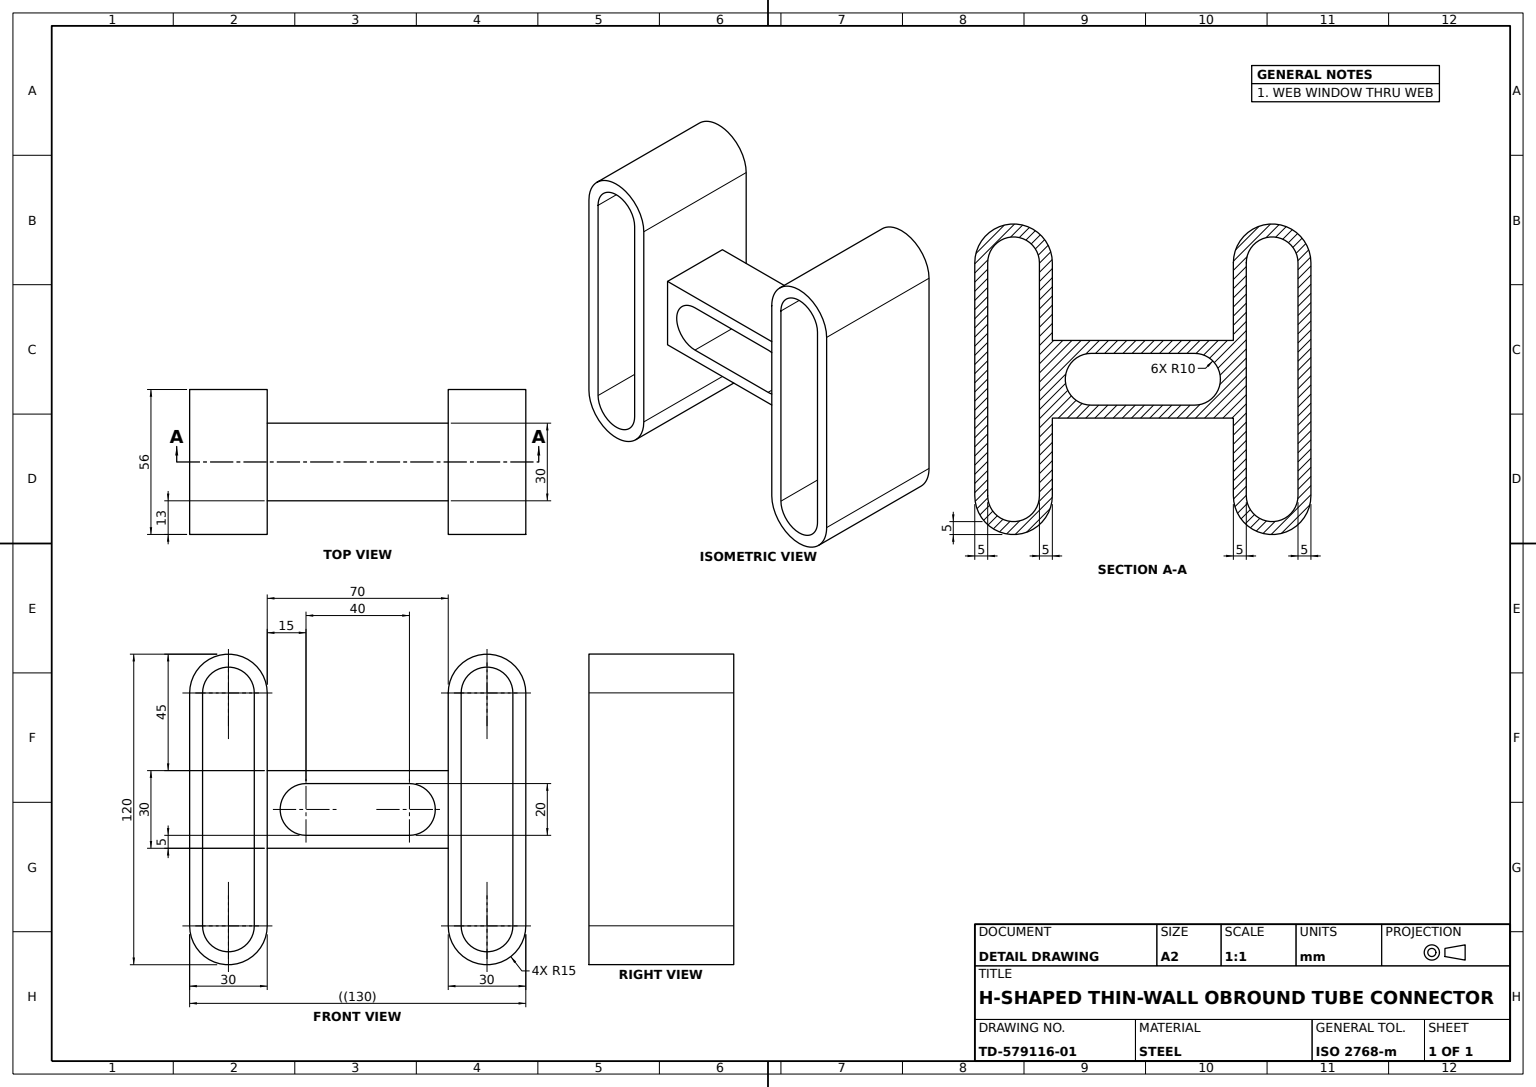
from build123d import *

# Parameters (mm, degrees)
CENTER_WEB_DEPTH     = 15
WEB_WINDOW_CUT_DEPTH = 80
SIDE_LOOP_DEPTH      = 28


with BuildPart() as part:
    # Center Web Profile → Center Web (new, symmetric)
    with BuildSketch(Plane.XY):
        Polygon((35, 0), (35, 15), (-35, 15), (-35, -15), (35, -15), align=None)
    extrude(amount=CENTER_WEB_DEPTH, both=True)

    # Web Window Profile 40x20 → Web Window Cut (cut)
    with BuildSketch(Plane.XY.offset(15)):
        with BuildLine():
            Line((-20, 10), (20, 10))
            ThreePointArc((20, 10), (30, 0), (20, -10))
            Line((20, -10), (-20, -10))
            ThreePointArc((-20, -10), (-30, 0), (-20, 10))
        make_face()
    extrude(amount=-WEB_WINDOW_CUT_DEPTH, mode=Mode.SUBTRACT)

    # Side Loop Profile → Side Loop (add, symmetric)
    with BuildSketch(Plane.XY):
        with BuildLine():
            Line((35, 0), (35, 45))
            ThreePointArc((35, 45), (50, 60), (65, 45))
            Line((65, 45), (65, -45))
            ThreePointArc((65, -45), (50, -60), (35, -45))
            Line((35, -45), (35, -15))
            Line((35, -15), (35, 0))
        make_face()
        with BuildLine():
            Line((60, 45), (60, -45))
            ThreePointArc((60, -45), (50, -55), (40, -45))
            Line((40, -45), (40, 45))
            ThreePointArc((40, 45), (50, 55), (60, 45))
        make_face(mode=Mode.SUBTRACT)
    side_loop = extrude(amount=SIDE_LOOP_DEPTH, both=True)

    # Side Loop Mirror: Side Loop across plane
    add(side_loop.mirror(Plane(origin=(0, 0, 0), x_dir=(0, 0, 1), z_dir=(1, 0, 0))))


solid = part.part
